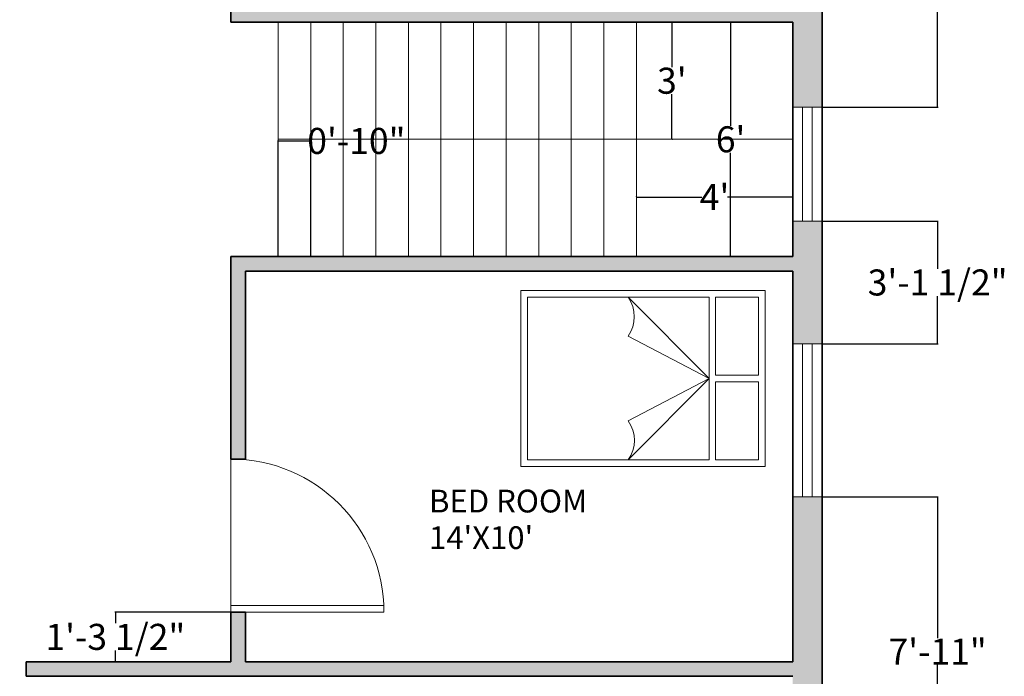
# Model space of a CAD drawing. Units: inches. Extents: x 638 to 1303, y 1 to 699.
# Tile 9 of 21: x 982 to 1284, y 207 to 409. Entities that reach past the tile are written whole.
import ezdxf

# ---------------------------------------------------------------- set-up
doc = ezdxf.new("R2010")
doc.units = ezdxf.units.IN
doc.header["$MEASUREMENT"] = 0
for name, color, linetype, lineweight in [('A-ANNO-DIMS', 2, 'Continuous', 18), ('A-AREA-IDEN', 7, 'Continuous', 18), ('A-DOOR', 4, 'Continuous', 18), ('A-FLOR-STRS', 7, 'Continuous', 18), ('A-GLAZ', 4, 'Continuous', 18), ('A-WALL', 7, 'Continuous', 35), ('Furniture', 7, 'Continuous', 15)]:
    doc.layers.add(name, color=color, linetype=linetype, lineweight=lineweight)
doc.layers.add('A-WALL-PATT', color=143, linetype='Continuous', lineweight=13, true_color=0x7aafdf)
doc.styles.get("Standard").update_dxf_attribs({"font": 'arial.ttf'})
doc.dimstyles.get("Standard").update_dxf_attribs({"dimtxt": 8, "dimasz": 0.18, "dimexe": 0.18, "dimexo": 0.0625, "dimgap": 0.09, "dimtad": 0, "dimtih": 1, "dimtoh": 1, "dimdec": 4, "dimzin": 0, "dimdsep": 46, "dimlunit": 3, "dimtxsty": 'Standard', "dimcen": 0.09, "dimadec": 0, "dimazin": 0, "dimtfac": 1, "dimtdec": 4, "dimtofl": 0, "dimtmove": 0, "dimatfit": 3, "dimfxl": 1, "dimtolj": 1, "dimtzin": 0, "dimarcsym": 0})

# ---------------------------------------------------------------- blocks, each defined once
blk = doc.blocks.new('*D6')
at = {"layer": 'A-ANNO-DIMS', "color": 0, "lineweight": -2, "transparency": 16777216}
for p, q in [((1211.87, 407.82), (1199.99, 407.82)), ((1200.17, 407.64), (1200.17, 375.99)), ((1200.17, 336), (1200.17, 367.64)), ((1211.87, 335.82), (1199.99, 335.82))]:
    blk.add_line(p, q, dxfattribs=at)
at = {"layer": 'A-ANNO-DIMS', "color": 0, "transparency": 16777216}
for points in [[(1200.14, 407.64), (1200.2, 407.64), (1200.17, 407.82)], [(1200.14, 336), (1200.2, 336), (1200.17, 335.82)]]:
    blk.add_solid(points, dxfattribs=at)
at = {"layer": 'Defpoints', "color": 0, "transparency": 16777216}
for p in [(1211.93, 407.82), (1200.17, 335.82), (1211.93, 335.82)]:
    blk.add_point(p, dxfattribs=at)
at = {"layer": 'A-ANNO-DIMS', "color": 0, "transparency": 16777216, "insert": (1200.17, 371.82), "char_height": 8, "attachment_point": 5}
blk.add_mtext("\\A1;6'", dxfattribs=at)
blk = doc.blocks.new('*D7')
at = {"layer": 'A-ANNO-DIMS', "color": 0, "lineweight": -2, "transparency": 16777216}
for p, q in [((1182.14, 407.64), (1182.14, 394)), ((1182.2, 407.82), (1182.32, 407.82)), ((1182.14, 372), (1182.14, 385.64)), ((1182.2, 371.82), (1182.32, 371.82))]:
    blk.add_line(p, q, dxfattribs=at)
at = {"layer": 'A-ANNO-DIMS', "color": 0, "transparency": 16777216}
for points in [[(1182.11, 407.64), (1182.17, 407.64), (1182.14, 407.82)], [(1182.11, 372), (1182.17, 372), (1182.14, 371.82)]]:
    blk.add_solid(points, dxfattribs=at)
at = {"layer": 'Defpoints', "color": 0, "transparency": 16777216}
for p in [(1182.14, 407.82), (1182.14, 407.82), (1182.14, 371.82)]:
    blk.add_point(p, dxfattribs=at)
at = {"layer": 'A-ANNO-DIMS', "color": 0, "transparency": 16777216, "insert": (1182.14, 389.82), "char_height": 8, "attachment_point": 5}
blk.add_mtext("\\A1;3'", dxfattribs=at)
blk = doc.blocks.new('*D8')
at = {"layer": 'A-ANNO-DIMS', "color": 0, "lineweight": -2, "transparency": 16777216}
for p, q in [((1171.24, 354.13), (1171.24, 354.25)), ((1171.42, 354.07), (1191.31, 354.07)), ((1219.06, 354.07), (1199.17, 354.07)), ((1219.24, 354.13), (1219.24, 354.25))]:
    blk.add_line(p, q, dxfattribs=at)
at = {"layer": 'A-ANNO-DIMS', "color": 0, "transparency": 16777216}
for points in [[(1171.42, 354.1), (1171.42, 354.04), (1171.24, 354.07)], [(1219.06, 354.1), (1219.06, 354.04), (1219.24, 354.07)]]:
    blk.add_solid(points, dxfattribs=at)
at = {"layer": 'Defpoints', "color": 0, "transparency": 16777216}
for p in [(1171.24, 354.07), (1171.24, 354.07), (1219.24, 354.07)]:
    blk.add_point(p, dxfattribs=at)
at = {"layer": 'A-ANNO-DIMS', "color": 0, "transparency": 16777216, "insert": (1195.24, 354.07), "char_height": 8, "attachment_point": 5}
blk.add_mtext("\\A1;4'", dxfattribs=at)
blk = doc.blocks.new('DOOR-SWING-47')
for p, q in [((45, 0), (45, 46.96)), ((47, 0), (47, 47)), ((0, 0), (47, 0))]:
    blk.add_line(p, q)
blk.add_arc((47, 0), 47, 90, 180)
blk = doc.blocks.new('WIN-47')
for p, q in [((47, 9), (0, 9)), ((0, 9), (0, 0)), ((47, 0), (47, 9)), ((0, 6), (47, 6)), ((0, 3), (47, 3)), ((0, 0), (47, 0))]:
    blk.add_line(p, q)
blk = doc.blocks.new('WIN-35')
for p, q in [((35, 9), (0, 9)), ((0, 9), (0, 0)), ((35, 0), (35, 9)), ((0, 6), (35, 6)), ((0, 3), (35, 3)), ((0, 0), (35, 0))]:
    blk.add_line(p, q)
blk = doc.blocks.new('*D48')
at = {"layer": 'A-ANNO-DIMS', "color": 0, "lineweight": -2, "transparency": 16777216}
for p, q in [((1228.3, 262), (1263.92, 262)), ((1263.74, 261.82), (1263.74, 218.52)), ((1263.74, 167.02), (1263.74, 210.31)), ((1228.3, 166.84), (1263.92, 166.84))]:
    blk.add_line(p, q, dxfattribs=at)
at = {"layer": 'A-ANNO-DIMS', "color": 0, "transparency": 16777216}
for points in [[(1263.71, 261.82), (1263.77, 261.82), (1263.74, 262)], [(1263.71, 167.02), (1263.77, 167.02), (1263.74, 166.84)]]:
    blk.add_solid(points, dxfattribs=at)
at = {"layer": 'Defpoints', "color": 0, "transparency": 16777216}
for p in [(1228.24, 262), (1263.74, 262), (1228.24, 166.84)]:
    blk.add_point(p, dxfattribs=at)
at = {"layer": 'A-ANNO-DIMS', "color": 0, "transparency": 16777216, "insert": (1263.74, 214.42), "char_height": 8, "attachment_point": 5}
blk.add_mtext('\\A1;7\'-11"', dxfattribs=at)
blk = doc.blocks.new('*D49')
at = {"layer": 'A-ANNO-DIMS', "color": 0, "lineweight": -2, "transparency": 16777216}
for p, q in [((1228.3, 346.66), (1263.92, 346.66)), ((1263.74, 346.48), (1263.74, 332.06)), ((1263.74, 309.18), (1263.74, 323.6)), ((1228.3, 309), (1263.92, 309))]:
    blk.add_line(p, q, dxfattribs=at)
at = {"layer": 'A-ANNO-DIMS', "color": 0, "transparency": 16777216}
for points in [[(1263.71, 346.48), (1263.77, 346.48), (1263.74, 346.66)], [(1263.71, 309.18), (1263.77, 309.18), (1263.74, 309)]]:
    blk.add_solid(points, dxfattribs=at)
at = {"layer": 'Defpoints', "color": 0, "transparency": 16777216}
for p in [(1228.24, 346.66), (1263.74, 346.66), (1228.24, 309)]:
    blk.add_point(p, dxfattribs=at)
at = {"layer": 'A-ANNO-DIMS', "color": 0, "transparency": 16777216, "insert": (1263.74, 327.83), "char_height": 8, "attachment_point": 5}
blk.add_mtext('\\A1;3\'-1 1/2"', dxfattribs=at)
blk = doc.blocks.new('*D50')
at = {"layer": 'A-ANNO-DIMS', "color": 0, "lineweight": -2, "transparency": 16777216}
for p, q in [((1228.3, 451.8), (1263.92, 451.8)), ((1263.74, 451.62), (1263.74, 420.91)), ((1263.74, 381.84), (1263.74, 412.56)), ((1228.3, 381.66), (1263.92, 381.66))]:
    blk.add_line(p, q, dxfattribs=at)
at = {"layer": 'A-ANNO-DIMS', "color": 0, "transparency": 16777216}
for points in [[(1263.71, 451.62), (1263.77, 451.62), (1263.74, 451.8)], [(1263.71, 381.84), (1263.77, 381.84), (1263.74, 381.66)]]:
    blk.add_solid(points, dxfattribs=at)
at = {"layer": 'Defpoints', "color": 0, "transparency": 16777216}
for p in [(1228.24, 451.8), (1263.74, 451.8), (1228.24, 381.66)]:
    blk.add_point(p, dxfattribs=at)
at = {"layer": 'A-ANNO-DIMS', "color": 0, "transparency": 16777216, "insert": (1263.74, 416.73), "char_height": 8, "attachment_point": 5}
blk.add_mtext('\\A1;5\'-10"', dxfattribs=at)
blk = doc.blocks.new('*D60')
at = {"layer": 'A-ANNO-DIMS', "color": 0, "lineweight": -2, "transparency": 16777216}
for p, q in [((1061.24, 335.88), (1061.24, 371.5)), ((1061.42, 371.32), (1071.06, 371.32)), ((1071.24, 335.88), (1071.24, 371.5)), ((1071.24, 371.32), (1071.42, 371.32))]:
    blk.add_line(p, q, dxfattribs=at)
at = {"layer": 'A-ANNO-DIMS', "color": 0, "transparency": 16777216}
for points in [[(1061.42, 371.35), (1061.42, 371.29), (1061.24, 371.32)], [(1071.06, 371.35), (1071.06, 371.29), (1071.24, 371.32)]]:
    blk.add_solid(points, dxfattribs=at)
at = {"layer": 'Defpoints', "color": 0, "transparency": 16777216}
for p in [(1071.24, 371.32), (1061.24, 335.82), (1071.24, 335.82)]:
    blk.add_point(p, dxfattribs=at)
at = {"layer": 'A-ANNO-DIMS', "color": 0, "transparency": 16777216, "insert": (1085.25, 371.32), "char_height": 8, "attachment_point": 5}
blk.add_mtext('\\A1;0\'-10"', dxfattribs=at)
blk = doc.blocks.new('*D64')
at = {"layer": 'A-ANNO-DIMS', "color": 0, "lineweight": -2, "transparency": 16777216}
for p, q in [((1046.68, 226.57), (1011.06, 226.57)), ((1011.24, 226.39), (1011.24, 223.17)), ((1011.24, 211.5), (1011.24, 214.71)), ((1046.68, 211.32), (1011.06, 211.32))]:
    blk.add_line(p, q, dxfattribs=at)
at = {"layer": 'A-ANNO-DIMS', "color": 0, "transparency": 16777216}
for points in [[(1011.21, 226.39), (1011.27, 226.39), (1011.24, 226.57)], [(1011.21, 211.5), (1011.27, 211.5), (1011.24, 211.32)]]:
    blk.add_solid(points, dxfattribs=at)
at = {"layer": 'Defpoints', "color": 0, "transparency": 16777216}
for p in [(1011.24, 226.57), (1046.74, 226.57), (1046.74, 211.32)]:
    blk.add_point(p, dxfattribs=at)
at = {"layer": 'A-ANNO-DIMS', "color": 0, "transparency": 16777216, "insert": (1011.24, 218.94), "char_height": 8, "attachment_point": 5}
blk.add_mtext('\\A1;1\'-3 1/2"', dxfattribs=at)

msp = doc.modelspace()

# ---------------------------------------------------------------- hatches: boundary and pattern name
at = {"layer": 'A-WALL-PATT'}
h = msp.add_hatch(color=256, dxfattribs=at)
h.dxf.hatch_style = 1
h.paths.add_polyline_path([(973.34524, 629.81895), (793.35541, 629.81895), (793.35541, 620.81895), (850.23798, 620.81895), (922.23798, 620.81895), (922.23798, 524.81895), (908.94335, 524.81895), (908.94335, 520.31895), (926.73798, 520.31895), (926.73798, 544.31895), (979.3571, 544.31895), (979.3571, 548.81895), (926.73798, 548.81895), (926.73798, 620.81895), (973.34524, 620.81895)])
h.paths.add_polyline_path([(758.35541, 629.81895), (697.23798, 629.81895), (697.23798, 586.77451), (706.23798, 586.77451), (706.23798, 620.81895), (758.35541, 620.81895)])
h.paths.add_polyline_path([(1075.85281, 629.81895), (1003.34524, 629.81895), (1003.34524, 620.81895), (1046.73798, 620.81895), (1046.73798, 560.81895), (1046.73798, 548.81895), (1026.3571, 548.81895), (1026.3571, 544.31895), (1046.73798, 544.31895), (1046.73798, 486.87457), (1051.23798, 486.87457), (1051.23798, 556.31895), (1162.89753, 556.31895), (1162.89753, 560.81895), (1051.23798, 560.81895), (1051.23798, 620.81895), (1075.85281, 620.81895)])
h.paths.add_polyline_path([(1228.23798, 629.81895), (1105.85281, 629.81895), (1105.85281, 620.81895), (1219.23798, 620.81895), (1219.23798, 560.81895), (1197.89753, 560.81895), (1197.89753, 556.31895), (1219.23798, 556.31895), (1219.23798, 498.80084), (1228.23798, 498.80084)])
h.paths.add_polyline_path([(1051.23798, 439.87457), (1046.73798, 439.87457), (1046.73798, 407.81895), (1219.23798, 407.81895), (1219.23798, 381.66175), (1228.23798, 381.66175), (1228.23798, 451.80084), (1219.23798, 451.80084), (1219.23798, 412.31895), (1051.23798, 412.31895)])
h.paths.add_polyline_path([(1228.23798, 346.66175), (1219.23798, 346.66175), (1219.23798, 335.81895), (1046.73798, 335.81895), (1046.73798, 273.56895), (1051.23798, 273.56895), (1051.23798, 331.31895), (1219.23798, 331.31895), (1219.23798, 308.99654), (1228.23798, 308.99654)])
h.paths.add_polyline_path([(1228.23798, 261.99654), (1219.23798, 261.99654), (1219.23798, 211.31895), (1051.23798, 211.31895), (1051.23798, 226.56895), (1046.73798, 226.56895), (1046.73798, 211.31895), (983.84714, 211.31895), (983.84714, 206.81895), (1219.23798, 206.81895), (1219.23798, 166.83987), (1228.23798, 166.83987)])
h.paths.add_polyline_path([(1228.23798, 119.83987), (1219.23798, 119.83987), (1219.23798, 50.81895), (1197.89277, 50.81895), (1197.89277, 41.81895), (1228.23798, 41.81895)])
h.paths.add_polyline_path([(1162.89277, 50.81895), (1069.02949, 50.81895), (1069.02949, 41.81895), (1162.89277, 41.81895)])
h.paths.add_polyline_path([(1010.02949, 50.81895), (941.89631, 50.81895), (917.77455, 50.81895), (917.77455, 41.81895), (941.89631, 41.81895), (1010.02949, 41.81895)])
h.paths.add_polyline_path([(882.77455, 50.81895), (854.73798, 50.81895), (854.73798, 145.50379), (850.23798, 145.50379), (850.23798, 50.81895), (793.49755, 50.81895), (793.49755, 41.81895), (882.77455, 41.81895)])
h.paths.add_polyline_path([(746.49755, 50.81895), (706.23798, 50.81895), (706.23798, 96.57416), (697.23798, 96.57416), (697.23798, 41.81895), (746.49755, 41.81895)])
h.paths.add_polyline_path([(706.23798, 206.81895), (714.01165, 206.81895), (714.01165, 211.31895), (706.23798, 211.31895), (706.23798, 251.21966), (697.23798, 251.21966), (697.23798, 143.57416), (706.23798, 143.57416)])
h.paths.add_polyline_path([(923.84714, 211.31895), (854.73798, 211.31895), (854.73798, 397.8313), (850.23798, 397.8313), (850.23798, 388.31895), (747.9539, 388.31895), (747.9539, 383.81895), (850.23798, 383.81895), (850.23798, 311.81895), (706.23798, 311.81895), (706.23798, 342.78787), (697.23798, 342.78787), (697.23798, 281.21966), (706.23798, 281.21966), (706.23798, 307.31895), (850.23798, 307.31895), (850.23798, 211.31895), (749.01165, 211.31895), (749.01165, 206.81895), (850.23798, 206.81895), (850.23798, 192.50379), (854.73798, 192.50379), (854.73798, 206.81895), (923.84714, 206.81895)])
h.paths.add_polyline_path([(706.23798, 434.70471), (697.23798, 434.70471), (697.23798, 372.78787), (706.23798, 372.78787), (706.23798, 383.81895), (712.9539, 383.81895), (712.9539, 388.31895), (706.23798, 388.31895)])
h.paths.add_polyline_path([(706.23798, 520.31895), (850.23798, 520.31895), (850.23798, 444.8313), (854.73798, 444.8313), (854.73798, 520.31895), (861.94335, 520.31895), (861.94335, 524.81895), (706.23798, 524.81895), (706.23798, 551.77451), (697.23798, 551.77451), (697.23798, 481.70471), (706.23798, 481.70471)])

# ---------------------------------------------------------------- linework, layer by layer
at = {"layer": 'A-FLOR-STRS'}
for p, q in [((1061.23798, 407.81895), (1061.23798, 335.81895)), ((1071.23798, 407.81895), (1071.23798, 335.81895)), ((1081.23798, 407.81895), (1081.23798, 335.81895)), ((1091.23798, 407.81895), (1091.23798, 335.81895)), ((1101.23798, 407.81895), (1101.23798, 335.81895)), ((1111.23798, 407.81895), (1111.23798, 335.81895)), ((1121.23798, 407.81895), (1121.23798, 335.81895)), ((1131.23798, 407.81895), (1131.23798, 335.81895)), ((1141.23798, 407.81895), (1141.23798, 335.81895)), ((1151.23798, 407.81895), (1151.23798, 335.81895)), ((1161.23798, 407.81895), (1161.23798, 335.81895)), ((1171.23798, 407.81895), (1171.23798, 335.81895)), ((1219.23798, 371.81895), (1061.23798, 371.81895))]:
    msp.add_line(p, q, dxfattribs=at)
at = {"layer": 'A-WALL'}
for p, q in [((1228.23798, 629.81895), (1228.23798, 41.81895)), ((1046.73798, 439.87457), (1046.73798, 407.81895)), ((1219.23798, 407.81895), (1046.73798, 407.81895)), ((1219.23798, 407.81895), (1219.23798, 335.81895)), ((1219.23798, 335.81895), (1046.73798, 335.81895)), ((1046.73798, 335.81895), (1046.73798, 273.56895)), ((1219.23798, 331.31895), (1051.23798, 331.31895)), ((1051.23798, 331.31895), (1051.23798, 273.56895)), ((1219.23798, 331.31895), (1219.23798, 211.31895)), ((1046.73798, 273.56895), (1051.23798, 273.56895)), ((1046.73798, 226.56895), (1051.23798, 226.56895)), ((1046.73798, 226.56895), (1046.73798, 211.31895)), ((1051.23798, 226.56895), (1051.23798, 211.31895)), ((1046.73798, 211.31895), (983.84714, 211.31895)), ((983.84714, 211.31895), (983.84714, 206.81895)), ((1219.23798, 211.31895), (1051.23798, 211.31895)), ((1219.23798, 206.81895), (983.84714, 206.81895))]:
    msp.add_line(p, q, dxfattribs=at)
at = {"layer": 'Furniture'}
for p, q in [((1193.57863, 298.31895), (1168.68062, 323.31895)), ((1193.57863, 323.31895), (1193.57863, 273.31895)), ((1195.57863, 323.31895), (1195.57863, 299.31895)), ((1168.68062, 311.31895), (1193.57863, 298.31895)), ((1193.57863, 298.31895), (1168.68062, 273.31895)), ((1168.68062, 285.31895), (1193.57863, 298.31895)), ((1195.57863, 299.31895), (1208.77632, 299.31895)), ((1195.57863, 297.31895), (1208.77632, 297.31895)), ((1195.57863, 297.31895), (1195.57863, 273.31895))]:
    msp.add_line(p, q, dxfattribs=at)
msp.add_lwpolyline([(1135.77632, 325.31895), (1135.77632, 271.31895), (1210.77632, 271.31895), (1210.77632, 325.31895)], close=True, dxfattribs=at)
for points in [[(1193.57863, 323.31895), (1137.77632, 323.31895), (1137.77632, 273.31895), (1193.57863, 273.31895)], [(1208.77632, 299.31895), (1208.77632, 323.31895), (1195.57863, 323.31895)], [(1195.57863, 273.31895), (1208.77632, 273.31895), (1208.77632, 297.31895)]]:
    msp.add_lwpolyline(points, dxfattribs=at)
for centre, radius, start, end in [((1160.18704, 317.31895), 10.39908, 324.761993, 35.238007), ((1160.53038, 279.31895), 10.12059, 323.640432, 36.359568)]:
    msp.add_arc(centre, radius, start, end, dxfattribs=at)

# ---------------------------------------------------------------- block references
at = {"layer": 'A-DOOR', "rotation": 270.0000000000002}
msp.add_blockref('DOOR-SWING-47', (1046.73803, 273.5693), dxfattribs=at)
at = {"layer": 'A-GLAZ'}
for name, p, rotation in [('WIN-35', (1219.23803, 381.66153), 270.0000000000009), ('WIN-47', (1219.23803, 308.99609), 270.000000000001)]:
    msp.add_blockref(name, p, dxfattribs=dict(at, rotation=rotation))

# ---------------------------------------------------------------- texts
at = {"layer": 'A-AREA-IDEN'}
for s, p in [('BED ROOM', (1107.56529, 257.16362)), ("14'X10'", (1107.56529, 245.91874))]:
    msp.add_text(s, height=7, dxfattribs=at).set_placement(p)

# ---------------------------------------------------------------- dimensions: what is measured, and where the dimension line sits
at = {"layer": 'A-ANNO-DIMS'}
for base, p1, p2, override, picture, middle in [((1263.73798, 451.80084), (1228.23798, 381.66175), (1228.23798, 451.80084), {"dimdec": 1, "dimlfac": 1, "dimrnd": 0, "dimzin": 1, "dimdsep": 46, "dimlunit": 4, "dimfrac": 2}, '*D50', (1263.73798, 416.7313)), ((1182.14007, 407.81895), (1182.14007, 371.81895), (1182.14007, 407.81895), {"dimclrd": 0, "dimclre": 0, "dimclrt": 0}, '*D7', (1182.14007, 389.81895)), ((1200.1736, 335.81895), (1211.93461, 407.81895), (1211.93461, 335.81895), {"dimclrd": 0, "dimclre": 0, "dimclrt": 0}, '*D6', (1200.1736, 371.81895)), ((1263.73798, 346.66175), (1228.23798, 308.99654), (1228.23798, 346.66175), {"dimdec": 1, "dimlfac": 1, "dimrnd": 0, "dimzin": 1, "dimdsep": 46, "dimlunit": 4, "dimfrac": 2}, '*D49', (1263.73798, 327.82915)), ((1263.73798, 261.99654), (1228.23798, 166.83987), (1228.23798, 261.99654), {"dimdec": 1, "dimlfac": 1, "dimrnd": 0, "dimzin": 1, "dimdsep": 46, "dimlunit": 4, "dimfrac": 2}, '*D48', (1263.73798, 214.4182)), ((1011.237979, 226.568947), (1046.737979, 211.318947), (1046.737979, 226.568947), {"dimdec": 1, "dimlfac": 1, "dimrnd": 0, "dimzin": 1, "dimdsep": 46, "dimlunit": 4, "dimfrac": 2}, '*D64', (1011.237979, 218.943947))]:
    dim = msp.add_linear_dim(base=base, p1=p1, p2=p2, angle=90, dimstyle='Standard', override=override, dxfattribs=at)
    dim.commit()
    dim.dimension.update_dxf_attribs({"geometry": picture, "text_midpoint": middle})
for base, p1, p2, override, picture, middle in [((1071.23798, 371.31895), (1061.23798, 335.81895), (1071.23798, 335.81895), {"dimdec": 1, "dimlfac": 1, "dimrnd": 0, "dimzin": 1, "dimdsep": 46, "dimlunit": 4, "dimfrac": 2}, '*D60', (1085.24877, 371.31895)), ((1171.23798, 354.06915), (1219.23798, 354.06915), (1171.23798, 354.06915), {"dimclrd": 0, "dimclre": 0, "dimclrt": 0}, '*D8', (1195.23798, 354.06915))]:
    dim = msp.add_linear_dim(base=base, p1=p1, p2=p2, dimstyle='Standard', override=override, dxfattribs=at)
    dim.commit()
    dim.dimension.update_dxf_attribs({"geometry": picture, "text_midpoint": middle})

doc.saveas('drawing.dxf')
